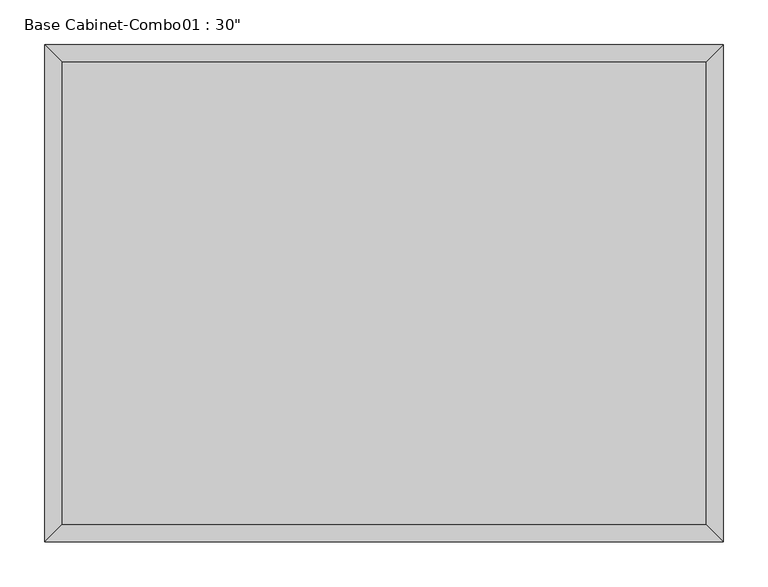
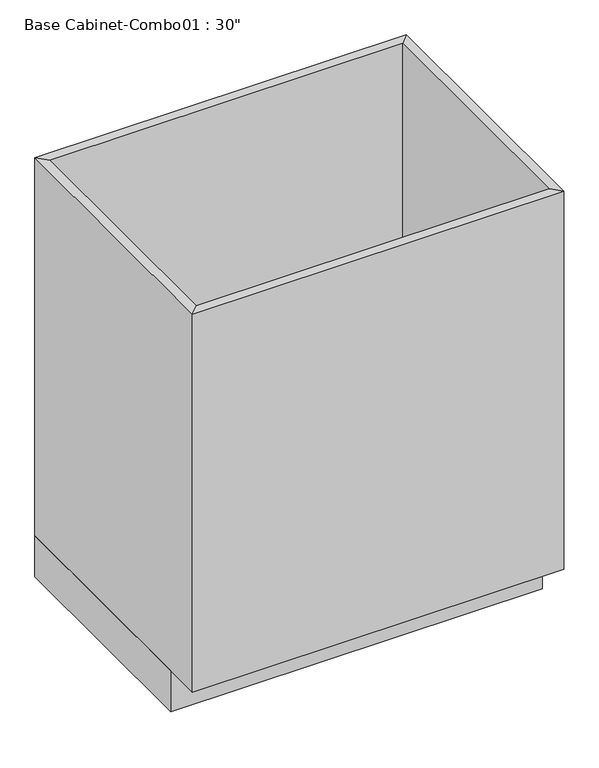
"""IFC4 building model written with IfcOpenShell, lengths in millimetres: furniture geometry."""

from ifc_helpers import new_model, si_unit, frame, origin, origin_with_axes, place, context, project, spatial, polyline, outline, extrude, faceted_brep, source, transform, mapped, element, save


def furniture_f87f75a4(model_context):
    return source(origin(), model_context, "Body", "SolidModel", [
        extrude(outline(polyline([(399.7377049, 0.0), (399.7377049, -482.6), (-362.2622951, -482.6), (-362.2622951, 0.0), (399.7377049, 0.0)])), origin_with_axes(), (0.0, 0.0, 1.0), 88.9),
        faceted_brep([(380.6877049, -539.75, 908.05), (380.6877049, -539.75, 88.9), (-343.2122951, -539.75, 88.9), (-343.2122951, -539.75, 908.05), (399.7377049, -558.8, 908.05), (-362.2622951, -558.8, 908.05), (399.7377049, -558.8, 88.9), (-362.2622951, -558.8, 88.9), (-343.2122951, -19.05, 88.9), (-343.2122951, -19.05, 908.05), (-362.2622951, 0.0, 908.05), (-362.2622951, 0.0, 88.9), (380.6877049, -19.05, 88.9), (380.6877049, -19.05, 908.05), (399.7377049, 0.0, 908.05), (399.7377049, 0.0, 88.9)], [[[0, 1, 2, 3]], [[4, 0, 3, 5]], [[6, 4, 5, 7]], [[1, 6, 7, 2]], [[3, 2, 8, 9]], [[5, 3, 9, 10]], [[7, 5, 10, 11]], [[2, 7, 11, 8]], [[9, 8, 12, 13]], [[10, 9, 13, 14]], [[11, 10, 14, 15]], [[8, 11, 15, 12]], [[13, 12, 1, 0]], [[14, 13, 0, 4]], [[15, 14, 4, 6]], [[12, 15, 6, 1]]]),
        extrude(outline(polyline([(380.6877049, -19.05), (380.6877049, -539.75), (-343.2122951, -539.75), (-343.2122951, -19.05), (380.6877049, -19.05)])), frame((0.0, 0.0, 88.9), z_axis=(0.0, 0.0, 1.0), x_axis=(1.0, 0.0, 0.0)), (0.0, 0.0, 1.0), 19.05),
    ])


if __name__ == "__main__":
    model = new_model("IFC4")
    model_context = context("Model", 3, world=origin())
    ifc_project = project(units=[si_unit("LENGTHUNIT", "METRE", prefix="MILLI")], contexts=[model_context])
    site = spatial("IfcSite", under=ifc_project)
    building = spatial("IfcBuilding", under=site)
    placement = place(None, origin())
    furniture_shape = furniture_f87f75a4(model_context)
    element("IfcFurniture", 1, ObjectType="Base Cabinet-Combo01 : 30\"", at=placement, inside=building, context=model_context, shape_type="MappedRepresentation", body=[
        mapped(furniture_shape, transform((0.0, 0.0, 0.0), x_axis=(1.0, 0.0, 0.0), y_axis=(0.0, 1.0, 0.0), z_axis=(0.0, 0.0, 1.0))),
    ])
    save(model, "model.ifc")

# Revit data of these elements
# Type "Base Cabinet-Combo01 : 30\""
#   Depth = 1' - 10"
#   Height = 2' - 11 3/4"
#   Toe Depth = 0' - 3"
#   Toe Height = 0' - 3 1/2"
#   Width = 2' - 6"
#   Default Elevation = 0
# Element 1 (IfcFurniture, "Base Cabinet-Combo01 : 30\"")
#   Materials on its faces: "Cabinet"
# Materials
#   "Cabinet": colour RGB 204 122 2, transparency 0
